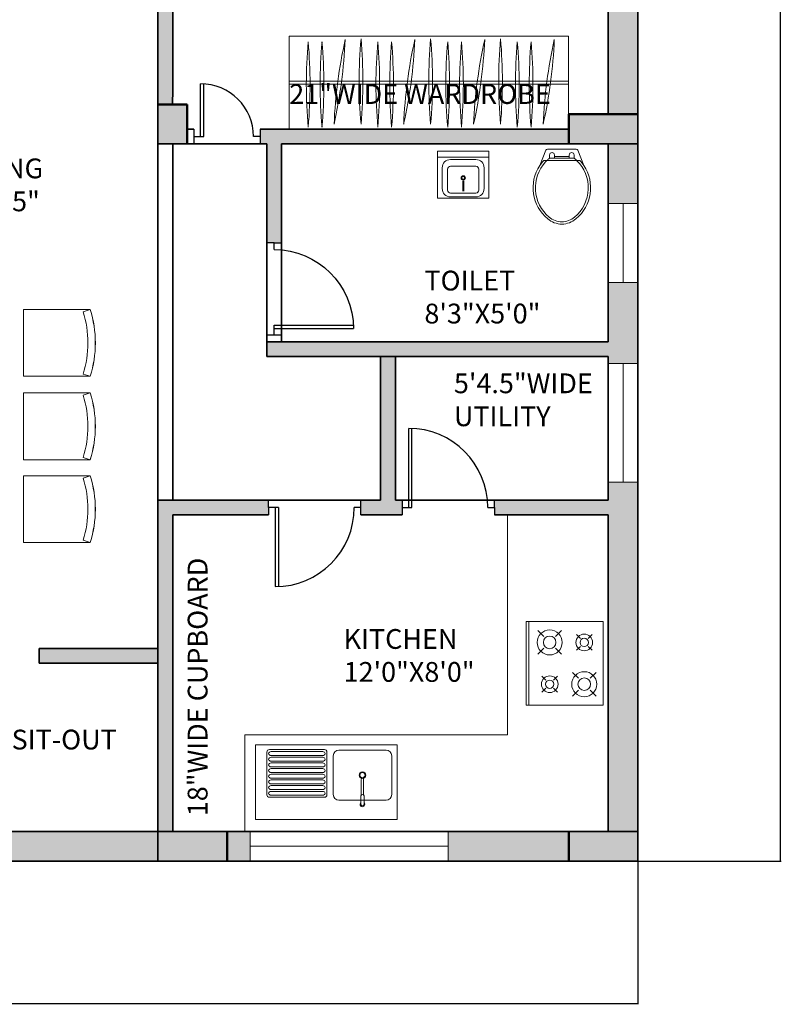
# Model space of a CAD drawing. Units: inches. Extents: x -28 to 485, y -861 to 54.
# Tile 4 of 14: x 254 to 485, y -861 to -563. Entities that reach past the tile are written whole.
import ezdxf

# ---------------------------------------------------------------- set-up
doc = ezdxf.new("R2010")
doc.units = ezdxf.units.IN
doc.header["$MEASUREMENT"] = 0
for name, color, linetype, lineweight in [('A-ANNO-DIMS', 2, 'Continuous', 18), ('A-ANNO-TEXT', 7, 'Continuous', 18), ('A-AREA-IDEN', 7, 'Continuous', 18), ('A-COLS', 7, 'Continuous', 50), ('A-COLS-PATT', 8, 'Continuous', 13), ('A-DOOR', 3, 'Continuous', 25), ('A-EQPM', 9, 'Continuous', 18), ('A-FLOR-CASE', 8, 'Continuous', 18), ('A-FLOR-FIXT', 9, 'Continuous', 18), ('A-FURN', 8, 'Continuous', 13), ('A-GLAZ', 4, 'Continuous', 18), ('A-WALL', 7, 'Continuous', 35), ('A-WALL-PATT', 34, 'Continuous', 13)]:
    doc.layers.add(name, color=color, linetype=linetype, lineweight=lineweight)
doc.styles.get("Standard").update_dxf_attribs({"font": 'arial.ttf'})
doc.dimstyles.get("Standard").update_dxf_attribs({"dimtxt": 0.18, "dimasz": 0.18, "dimexe": 0.18, "dimexo": 0.0625, "dimgap": 0.09, "dimtad": 0, "dimtih": 1, "dimtoh": 1, "dimdec": 0, "dimzin": 0, "dimdsep": 46, "dimlunit": 3, "dimtxsty": 'Standard', "dimcen": 0.09, "dimadec": 0, "dimazin": 0, "dimtfac": 1, "dimtdec": 0, "dimtofl": 0, "dimtmove": 0, "dimatfit": 3, "dimfxl": 1, "dimtolj": 1, "dimtzin": 0, "dimarcsym": 0})

# ---------------------------------------------------------------- blocks, each defined once
blk = doc.blocks.new('М14 600х655')
for p, q in [((-655, 600), (-655, 0)), ((-655, 600), (-655, 0)), ((-655, 0), (-655, 600)), ((0, 600), (-655, 600)), ((0, 525), (-655, 525)), ((0, 0), (0, 600)), ((-596, 388), (-596, 121)), ((-165, 494), (-490, 494)), ((-165, 408), (-490, 408)), ((-59, 121), (-59, 388)), ((-528, 370), (-528, 103)), ((-127, 103), (-127, 370)), ((-334, 87), (-334, 220)), ((-321, 87), (-321, 220)), ((-655, 0), (-655, 0)), ((-655, 0), (-655, 0)), ((-655, 0), (0, 0)), ((-655, 0), (0, 0)), ((-490, 65), (-165, 65)), ((-490, 15), (-165, 15))]:
    blk.add_line(p, q)
for radius in [27.6, 19.3]:
    blk.add_circle((-327, 259), radius)
for centre, radius, start, end in [((-490, 388), 106, 90, 180), ((-490, 370), 38.2, 90, 180), ((-165, 388), 106, 0, 90), ((-165, 370), 38.2, 0, 90), ((-490, 121), 106, 180, 270), ((-490, 103), 38.2, 180, 270), ((-165, 121), 106, 270, 0), ((-165, 103), 38.2, 270, 0)]:
    blk.add_arc(centre, radius, start, end)
blk = doc.blocks.new('WARDROBE-HANGING')
for p, q in [((84.7, 28.23), (0, 28.23)), ((0, 28.23), (0, 0)), ((84.7, 28.23), (84.7, 0)), ((84.7, 14.59), (0, 14.59)), ((84.7, 13.65), (0, 13.65)), ((84.7, 0), (0, 0))]:
    blk.add_line(p, q)
for centre, start, end in [((-131.46, 33.65), 347.508, 357.5023), ((162.01, -4.96), 167.508, 177.5023), ((169.76, 14.46), 175.0028, 184.9972), ((-126.23, 14.46), 355.0028, 4.9972), ((-110.36, 33.65), 347.508, 357.5023), ((183.11, -4.96), 167.508, 177.5023), ((190.86, 14.46), 175.0028, 184.9972), ((-105.13, 14.46), 355.0028, 4.9972), ((204.29, -4.96), 167.508, 177.5023), ((-89.17, 33.65), 347.508, 357.5023), ((212.05, 14.46), 175.0028, 184.9972), ((-83.95, 14.46), 355.0028, 4.9972), ((225.4, -4.96), 167.508, 177.5023), ((-68.07, 33.65), 347.508, 357.5023), ((153.74, 13.55), 175.0028, 184.9972), ((-142.25, 13.55), 355.0028, 4.9972), ((157.93, 13.55), 175.0028, 184.9972), ((-138.07, 13.55), 355.0028, 4.9972), ((174.85, 13.55), 175.0028, 184.9972), ((-121.15, 13.55), 355.0028, 4.9972), ((179.03, 13.55), 175.0028, 184.9972), ((-116.97, 13.55), 355.0028, 4.9972), ((196.03, 13.55), 175.0028, 184.9972), ((-99.97, 13.55), 355.0028, 4.9972), ((200.21, 13.55), 175.0028, 184.9972), ((-95.78, 13.55), 355.0028, 4.9972), ((217.13, 13.55), 175.0028, 184.9972), ((-78.86, 13.55), 355.0028, 4.9972), ((221.31, 13.55), 175.0028, 184.9972), ((-74.68, 13.55), 355.0028, 4.9972)]:
    blk.add_arc(centre, 148.56, start, end)
blk = doc.blocks.new('WC-FLOOR-MOUNTED')
for p, q in [((3.27, 19.35), (4.23, 19.35)), ((4.23, 19.35), (8.71, 19.35)), ((13.2, 19.35), (8.71, 19.35)), ((13.2, 19.35), (14.16, 19.35))]:
    blk.add_line(p, q)
for points in [[(8.71, 22.81), (4.36, 22.81, 0.31031), (3.82, 22.44), (2.03, 17.79, 0.209071)], [(5.01, 20.04), (5.01, 21, -1), (6.47, 21), (6.47, 20.5)], [(8.71, 22.81), (13.07, 22.81, -0.31031), (13.6, 22.44), (15.39, 17.79, -0.209071)], [(12.41, 20.04), (12.41, 21, 1), (10.96, 21), (10.96, 20.5)], [(3.77, 18.89, 0.431639), (4.86, 2.17, 0.162618), (8.71, 0.68, 0.470877)], [(3.27, 19.35, 0.040937), (2.03, 17.79, 0.163732)], [(4.23, 19.35, 0.014165), (3.77, 18.89, 0.162618)], [(5.01, 20.04, 0.022712), (4.23, 19.35, 0.162618)], [(8.71, 20.04), (5.01, 20.04, 0.022712)], [(8.71, 20.04), (12.41, 20.04, -0.476108)], [(13.2, 19.35, -0.448546), (12.57, 2.17, -0.162618), (8.71, 0.68, -0.470877)], [(12.41, 20.04, -0.022712), (13.2, 19.35, -0.162618)], [(14.16, 19.35, -0.040937), (15.39, 17.79, -0.163732)], [(2.03, 17.79, 0.383919), (4.43, 1.64, 0.163732), (8.71, 0, 0.359733)], [(15.39, 17.79, -0.383919), (13, 1.64, -0.163732), (8.71, 0, -0.359733)]]:
    blk.add_lwpolyline(points, format="xyb")
for points in [[(10.96, 20.5), (6.47, 20.5)], [(6.47, 20.5), (6.47, 20.04)], [(10.96, 20.5), (10.96, 20.04)]]:
    blk.add_lwpolyline(points)
blk = doc.blocks.new('COOKTOP-FOUR-BURNER')
for p, q in [((0, 0), (0, 25.33)), ((0, 25.33), (23.39, 25.33)), ((0.84, 0), (0.84, 25.33)), ((23.39, 0), (23.39, 25.33)), ((5.39, 20.79), (3.59, 22.58)), ((8.97, 20.79), (10.76, 22.58)), ((16.47, 20.19), (15.27, 21.39)), ((18.85, 20.19), (20.05, 21.39)), ((5.39, 17.21), (3.59, 15.42)), ((8.97, 17.21), (10.76, 15.42)), ((16.47, 17.8), (15.27, 16.61)), ((18.85, 17.8), (20.05, 16.61)), ((15.87, 8.12), (14.08, 9.91)), ((19.45, 8.12), (21.24, 9.91)), ((5.98, 7.53), (4.79, 8.72)), ((8.37, 7.53), (9.57, 8.72)), ((5.98, 5.14), (4.79, 3.94)), ((8.37, 5.14), (9.57, 3.94)), ((15.87, 4.54), (14.08, 2.75)), ((19.45, 4.54), (21.24, 2.75)), ((0, 0), (23.39, 0))]:
    blk.add_line(p, q)
for centre, radius in [((7.18, 19), 3.8), ((17.66, 19), 2.53), ((17.66, 6.33), 3.8), ((7.18, 6.33), 2.53)]:
    blk.add_circle(centre, radius)
for centre, radius, start, end in [((7.18, 19), 1.9, 90, 270), ((7.18, 19), 1.9, 270, 90), ((17.66, 19), 1.27, 90, 270), ((17.66, 19), 1.27, 270, 90), ((7.18, 6.33), 1.27, 90, 270), ((7.18, 6.33), 1.27, 270, 90), ((17.66, 6.33), 1.9, 90, 270), ((17.66, 6.33), 1.9, 270, 90)]:
    blk.add_arc(centre, radius, start, end)
blk = doc.blocks.new('CHAIR-DINING')
for p, q in [((20.22, 20.23), (18.08, 19.55)), ((20.22, 0), (18.08, 0.68))]:
    blk.add_line(p, q)
blk.add_lwpolyline([(20.23, 0), (0, 0), (0, 20.23), (20.23, 20.23, -0.153703), (20.23, 0)], format="xyb")
for radius in [31.13, 33.37]:
    blk.add_arc((-11.59, 10.12), radius, 342.3544, 17.6456)
blk = doc.blocks.new('DOOR-SWING-24')
for p, q in [((2, 2.25), (2, 26.25)), ((3, 2.25), (3, 26.25)), ((0, 4.5), (0, 0)), ((28, 2.25), (28, 4.5)), ((0, 2.25), (2, 2.25)), ((2, 2.25), (3, 2.25)), ((26, 2.25), (28, 2.25)), ((28, 2.25), (28, 0))]:
    blk.add_line(p, q)
blk.add_arc((2, 2.25), 24, 0, 90)
blk = doc.blocks.new('DOOR-SWING-KITCHEN')
for p, q in [((0, 24), (0, 26.25)), ((2, 24), (0, 24)), ((0, 24), (0, 21.75)), ((2, 24), (2, 0)), ((3, 24), (2, 24)), ((3, 24), (3, 0)), ((28, 24), (26, 24)), ((28, 21.75), (28, 26.25))]:
    blk.add_line(p, q)
blk.add_arc((2, 24), 24, 270, 0)
blk = doc.blocks.new('WINDOW-60IN')
for p, q in [((0, 60), (0, 0)), ((9, 60), (0, 60)), ((4.5, 60), (4.5, 0)), ((9, 0), (9, 60)), ((0, 0), (9, 0))]:
    blk.add_line(p, q)
blk = doc.blocks.new('WINDOW-36IN')
for p, q in [((0, 36), (0, 0)), ((9, 36), (0, 36)), ((4.5, 36), (4.5, 0)), ((9, 0), (9, 36)), ((0, 0), (9, 0))]:
    blk.add_line(p, q)
blk = doc.blocks.new('WINDOW-24IN')
for p, q in [((0, 24), (0, 0)), ((9, 24), (0, 24)), ((4.5, 24), (4.5, 0)), ((9, 0), (9, 24)), ((9, 0), (0, 0))]:
    blk.add_line(p, q)
blk = doc.blocks.new('*D52')
at = {"layer": 'A-ANNO-DIMS', "color": 0, "lineweight": -2, "transparency": 16777216}
for p, q in [((15.28, -817.93), (15.28, -861.3)), ((441.28, -817.93), (441.28, -861.3)), ((15.46, -861.12), (227.99, -861.12)), ((441.1, -861.12), (228.58, -861.12))]:
    blk.add_line(p, q, dxfattribs=at)
at = {"layer": 'A-ANNO-DIMS', "color": 0, "transparency": 16777216}
for points in [[(15.46, -861.09), (15.46, -861.15), (15.28, -861.12)], [(441.1, -861.09), (441.1, -861.15), (441.28, -861.12)]]:
    blk.add_solid(points, dxfattribs=at)
at = {"layer": 'Defpoints', "color": 0, "transparency": 16777216}
for p in [(15.28, -817.87), (441.28, -817.87), (441.28, -861.12)]:
    blk.add_point(p, dxfattribs=at)
at = {"layer": 'A-ANNO-DIMS', "color": 0, "transparency": 16777216, "insert": (228.28, -861.12), "char_height": 0.18, "attachment_point": 5}
blk.add_mtext('\\A1;426', dxfattribs=at)
blk = doc.blocks.new('*D53')
at = {"layer": 'A-ANNO-DIMS', "color": 0, "lineweight": -2, "transparency": 16777216}
for p, q in [((441.35, 10.13), (484.71, 10.13)), ((484.53, 9.95), (484.53, -403.68)), ((484.53, -817.69), (484.53, -404.05)), ((441.35, -817.87), (484.71, -817.87))]:
    blk.add_line(p, q, dxfattribs=at)
at = {"layer": 'A-ANNO-DIMS', "color": 0, "transparency": 16777216}
for points in [[(484.5, 9.95), (484.56, 9.95), (484.53, 10.13)], [(484.5, -817.69), (484.56, -817.69), (484.53, -817.87)]]:
    blk.add_solid(points, dxfattribs=at)
at = {"layer": 'Defpoints', "color": 0, "transparency": 16777216}
for p in [(441.28, 10.13), (441.28, -817.87), (484.53, -817.87)]:
    blk.add_point(p, dxfattribs=at)
at = {"layer": 'A-ANNO-DIMS', "color": 0, "transparency": 16777216, "insert": (484.53, -403.87), "char_height": 0.18, "attachment_point": 5}
blk.add_mtext('\\A1;828', dxfattribs=at)

msp = doc.modelspace()

# ---------------------------------------------------------------- hatches: boundary and pattern name
at = {"layer": 'A-COLS-PATT'}
h = msp.add_hatch(color=256, dxfattribs=at)
h.dxf.hatch_style = 1
h.paths.add_polyline_path([(441.285, -591.367), (420.285, -591.367), (420.285, -595.867), (420.285, -600.367), (441.285, -600.367)])
h.paths.add_polyline_path([(304.691, -588.367), (295.785, -588.367), (295.785, -600.367), (304.691, -600.367)])
h.paths.add_polyline_path([(160.785, -588.367), (151.785, -588.367), (151.785, -600.367), (160.785, -600.367)])
h.paths.add_polyline_path([(36.285, -591.367), (24.285, -591.367), (15.285, -591.367), (15.285, -600.367), (36.285, -600.367)])
h.paths.add_polyline_path([(36.285, -808.867), (15.285, -808.867), (15.285, -817.867), (36.285, -817.867)])
h.paths.add_polyline_path([(160.785, -808.867), (139.785, -808.867), (139.785, -817.867), (160.785, -817.867)])
h.paths.add_polyline_path([(316.785, -808.867), (295.785, -808.867), (295.785, -817.867), (316.785, -817.867)])
h.paths.add_polyline_path([(441.285, -808.867), (420.285, -808.867), (420.285, -817.867), (441.285, -817.867)])
h.paths.add_polyline_path([(36.285, -442.867), (15.285, -442.867), (15.285, -451.867), (36.285, -451.867)])
h.paths.add_polyline_path([(160.785, -442.867), (139.785, -442.867), (139.785, -451.867), (160.785, -451.867)])
h.paths.add_polyline_path([(316.785, -442.867), (295.785, -442.867), (295.785, -451.867), (316.785, -451.867)])
h.paths.add_polyline_path([(441.285, -442.867), (420.285, -442.867), (420.285, -451.867), (441.285, -451.867)])
at = {"layer": 'A-WALL-PATT'}
h = msp.add_hatch(color=256, dxfattribs=at)
h.dxf.hatch_style = 1
h.paths.add_polyline_path([(160.785, -808.867), (160.785, -817.867), (295.785, -817.867), (295.785, -808.867)])
h.paths.add_polyline_path([(316.785, -817.867), (323.776, -817.867), (323.776, -808.867), (316.785, -808.867)])
h.paths.add_polyline_path([(420.285, -817.867), (420.285, -808.867), (383.776, -808.867), (383.776, -817.867)])
h.paths.add_polyline_path([(432.285, -808.867), (441.285, -808.867), (441.285, -702.966), (432.285, -702.966), (432.285, -708.367), (397.785, -708.367), (397.785, -710.617), (397.785, -712.867), (432.285, -712.867)])
h.paths.add_polyline_path([(300.285, -712.867), (329.285, -712.867), (329.285, -710.617), (329.285, -708.367), (295.785, -708.367), (295.785, -808.867), (300.285, -808.867)])
h.paths.add_polyline_path([(160.785, -698.867), (158.535, -698.867), (156.285, -698.867), (156.285, -808.867), (160.785, -808.867)])
h.paths.add_polyline_path([(36.285, -808.867), (36.285, -817.867), (79.721, -817.867), (79.721, -808.867)])
h.paths.add_polyline_path([(15.285, -808.867), (24.285, -808.867), (24.285, -739.09), (15.285, -739.09)])
h.paths.add_polyline_path([(24.285, -640.781), (15.285, -640.781), (15.285, -679.09), (24.285, -679.09), (24.285, -664.867), (89.285, -664.867), (89.285, -662.617), (89.285, -660.367), (24.285, -660.367)])
h.paths.add_polyline_path([(15.285, -616.781), (24.285, -616.781), (24.285, -600.367), (15.285, -600.367)])
h.paths.add_polyline_path([(36.285, -595.867), (36.285, -600.367), (123.285, -600.367), (123.285, -660.367), (117.285, -660.367), (117.285, -664.867), (156.285, -664.867), (156.285, -670.867), (160.785, -670.867), (160.785, -660.367), (127.785, -660.367), (127.785, -600.367), (129.785, -600.367), (129.785, -598.117), (129.785, -595.867)])
h.paths.add_polyline_path([(367.785, -664.867), (363.285, -664.867), (363.285, -708.367), (357.285, -708.367), (357.285, -712.867), (369.785, -712.867), (369.785, -708.367), (367.785, -708.367)])
h.paths.add_polyline_path([(432.285, -664.867), (432.285, -666.966), (441.285, -666.966), (441.285, -642.367), (432.285, -642.367), (432.285, -660.367), (328.785, -660.367), (328.785, -664.867), (363.285, -664.867)])
h.paths.add_polyline_path([(333.285, -600.367), (420.285, -600.367), (420.285, -595.867), (326.785, -595.867), (326.785, -600.367), (328.785, -600.367), (328.785, -630.367), (331.035, -630.367), (333.285, -630.367)])
h.paths.add_polyline_path([(441.285, -600.367), (432.285, -600.367), (432.285, -618.367), (441.285, -618.367)])
h.paths.add_polyline_path([(432.285, -591.367), (441.285, -591.367), (441.285, -547.793), (432.285, -547.793)])
h.paths.add_polyline_path([(295.785, -588.367), (300.238, -588.367), (300.285, -583.867), (300.285, -451.867), (295.785, -451.867)])
h.paths.add_polyline_path([(420.285, -451.867), (420.285, -442.867), (316.785, -442.867), (316.785, -451.867)])
h.paths.add_polyline_path([(432.285, -487.793), (441.285, -487.793), (441.285, -451.867), (432.285, -451.867)])
h.paths.add_polyline_path([(432.285, -442.867), (441.285, -442.867), (441.285, -364.867), (432.285, -364.867)])
h.paths.add_polyline_path([(261.785, -451.867), (261.785, -447.367), (261.785, -444.758), (261.785, -442.867), (160.785, -442.867), (160.785, -451.867)])
h.paths.add_polyline_path([(139.785, -451.867), (139.785, -442.867), (36.285, -442.867), (36.285, -451.867)])
h.paths.add_polyline_path([(15.285, -491.617), (24.285, -491.617), (24.285, -451.867), (15.285, -451.867)])
h.paths.add_polyline_path([(24.285, -551.617), (15.285, -551.617), (15.285, -591.367), (24.285, -591.367)])
h.paths.add_polyline_path([(160.785, -451.867), (156.285, -451.867), (156.285, -588.367), (160.785, -588.367)])
h.paths.add_polyline_path([(139.785, -364.867), (139.785, -355.867), (36.285, -355.867), (36.285, -364.867)])
h.paths.add_polyline_path([(24.285, -364.867), (15.285, -364.867), (15.285, -373.867), (24.285, -373.867)])
h.paths.add_polyline_path([(15.285, -433.867), (15.285, -442.867), (24.285, -442.867), (24.285, -433.867)])
h.paths.add_polyline_path([(261.785, -364.867), (261.785, -360.367), (261.785, -355.867), (160.785, -355.867), (160.785, -364.867)])
h.paths.add_polyline_path([(295.785, -355.867), (289.785, -355.867), (289.785, -364.867), (295.785, -364.867)])
h.paths.add_polyline_path([(295.785, -355.867), (300.285, -355.867), (300.285, -259.867), (333.285, -259.867), (333.285, -257.617), (333.285, -255.367), (300.285, -255.367), (300.285, -207.367), (295.785, -207.367)])
h.paths.add_polyline_path([(420.285, -364.867), (420.285, -355.867), (316.785, -355.867), (316.785, -364.867)])
h.paths.add_polyline_path([(24.285, -311.192), (15.285, -311.192), (15.285, -355.867), (24.285, -355.867)])
h.paths.add_polyline_path([(24.285, -211.867), (54.144, -211.867), (54.144, -207.367), (24.285, -207.367), (24.285, -187.772), (15.285, -187.772), (15.285, -251.192), (24.285, -251.192)])
h.paths.add_polyline_path([(82.144, -207.367), (82.144, -209.617), (82.144, -211.867), (127.785, -211.867), (127.785, -147.367), (129.785, -147.367), (129.785, -145.117), (129.785, -142.867), (36.285, -142.867), (36.285, -147.367), (123.285, -147.367), (123.285, -207.367)])
h.paths.add_polyline_path([(160.785, -207.367), (156.285, -207.367), (156.285, -355.867), (160.785, -355.867)])
h.paths.add_polyline_path([(24.285, 1.133), (15.285, 1.133), (15.285, -54.408), (24.285, -54.408)])
h.paths.add_polyline_path([(36.285, 10.133), (36.285, 1.133), (70.235, 1.133), (70.235, 10.133)])
h.paths.add_polyline_path([(15.285, -138.367), (24.285, -138.367), (24.285, -114.408), (15.285, -114.408)])
h.paths.add_polyline_path([(24.285, -147.367), (15.285, -147.367), (15.285, -163.772), (24.285, -163.772)])
h.paths.add_polyline_path([(156.285, -130.867), (160.785, -130.867), (160.785, 1.133), (156.285, 1.133)])
h.paths.add_polyline_path([(130.235, 1.133), (139.785, 1.133), (139.785, 10.133), (130.235, 10.133)])
h.paths.add_polyline_path([(316.785, 10.133), (316.785, 1.133), (328.097, 1.133), (328.097, 10.133)])
h.paths.add_polyline_path([(300.285, 1.133), (295.785, 1.133), (295.785, -130.867), (300.285, -130.867)])
h.paths.add_polyline_path([(420.285, -147.367), (420.285, -142.867), (326.785, -142.867), (326.785, -145.117), (326.785, -147.367), (328.785, -147.367), (328.785, -177.367), (331.035, -177.367), (333.285, -177.367), (333.285, -147.367)])
h.paths.add_polyline_path([(333.285, -207.367), (333.285, -205.367), (328.785, -205.367), (328.785, -211.867), (363.285, -211.867), (363.285, -255.367), (361.285, -255.367), (361.285, -259.867), (369.785, -259.867), (369.785, -255.367), (367.785, -255.367), (367.785, -211.867), (432.285, -211.867), (432.285, -214.893), (441.285, -214.893), (441.285, -188.008), (432.285, -188.008), (432.285, -207.367)])
h.paths.add_polyline_path([(441.285, -250.893), (432.285, -250.893), (432.285, -255.367), (397.785, -255.367), (397.785, -257.617), (397.785, -259.867), (432.285, -259.867), (432.285, -355.867), (441.285, -355.867)])
h.paths.add_polyline_path([(432.285, -138.367), (441.285, -138.367), (441.285, -115.099), (432.285, -115.099)])
h.paths.add_polyline_path([(441.285, -147.367), (432.285, -147.367), (432.285, -164.008), (441.285, -164.008)])
h.paths.add_polyline_path([(420.285, 1.133), (420.285, 10.133), (388.097, 10.133), (388.097, 1.133)])
h.paths.add_polyline_path([(432.285, -55.099), (441.285, -55.099), (441.285, 1.133), (432.285, 1.133)])
h = msp.add_hatch(color=256, dxfattribs=at)
h.dxf.hatch_style = 1
h.paths.add_polyline_path([(196.785, -58.867), (160.785, -58.867), (160.785, -63.367), (196.785, -63.367)])
h.paths.add_polyline_path([(295.785, -58.867), (259.785, -58.867), (259.785, -63.367), (295.785, -63.367)])
h.paths.add_polyline_path([(196.785, -753.367), (160.785, -753.367), (160.785, -757.867), (196.785, -757.867)])
h.paths.add_polyline_path([(295.785, -753.367), (259.785, -753.367), (259.785, -757.867), (295.785, -757.867)])

# ---------------------------------------------------------------- linework, layer by layer
at = {"layer": 'A-COLS'}
for p, q in [((304.691, -588.367), (295.785, -588.367)), ((304.691, -600.367), (304.691, -588.367)), ((420.285, -595.867), (420.285, -591.367)), ((420.285, -591.367), (441.285, -591.367)), ((420.285, -600.367), (420.285, -595.867)), ((316.785, -808.867), (316.785, -817.867)), ((420.285, -808.867), (420.285, -817.867))]:
    msp.add_line(p, q, dxfattribs=at)
at = {"layer": 'A-DOOR'}
for p, q in [((308.691, -598.117), (308.691, -582.117)), ((309.691, -598.117), (309.691, -582.117)), ((306.691, -595.867), (306.691, -600.367)), ((326.785, -595.867), (326.785, -600.367)), ((306.691, -598.117), (308.691, -598.117)), ((308.691, -598.117), (309.691, -598.117)), ((326.785, -598.117), (324.785, -598.117))]:
    msp.add_line(p, q, dxfattribs=at)
msp.add_arc((308.691, -598.211), 16.094, 0.33541, 90, dxfattribs=at)
at = {"layer": 'A-FLOR-CASE'}
for p, q in [((401.695, -712.867), (401.695, -779.545)), ((401.695, -779.545), (322.083, -779.545)), ((322.083, -779.545), (322.083, -808.867))]:
    msp.add_line(p, q, dxfattribs=at)
at = {"layer": 'A-FLOR-FIXT'}
for p, q in [((368.283, -782.631), (325.404, -782.631)), ((325.404, -782.631), (325.404, -805.296)), ((328.806, -797.721), (328.806, -784.819)), ((346.232, -784.037), (329.587, -784.037)), ((337.91, -784.659), (330.057, -784.659)), ((337.91, -784.659), (345.762, -784.659)), ((347.014, -797.721), (347.014, -784.819)), ((364.954, -784.208), (350.618, -784.208)), ((368.283, -782.631), (368.283, -805.296)), ((337.91, -785.831), (330.057, -785.831)), ((337.91, -786.38), (330.057, -786.38)), ((337.91, -787.552), (330.057, -787.552)), ((337.91, -788.101), (330.057, -788.101)), ((337.91, -785.831), (345.762, -785.831)), ((337.91, -786.38), (345.762, -786.38)), ((337.91, -787.552), (345.762, -787.552)), ((337.91, -788.101), (345.762, -788.101)), ((348.93, -785.896), (348.93, -797.675)), ((366.642, -797.675), (366.642, -785.896)), ((337.91, -789.273), (330.057, -789.273)), ((337.91, -789.821), (330.057, -789.821)), ((337.91, -790.993), (330.057, -790.993)), ((337.91, -789.273), (345.762, -789.273)), ((337.91, -789.821), (345.762, -789.821)), ((337.91, -790.993), (345.762, -790.993)), ((337.91, -791.542), (330.057, -791.542)), ((337.91, -792.714), (330.057, -792.714)), ((337.91, -793.263), (330.057, -793.263)), ((337.91, -791.542), (345.762, -791.542)), ((337.91, -792.714), (345.762, -792.714)), ((337.91, -793.263), (345.762, -793.263)), ((337.91, -794.435), (330.057, -794.435)), ((337.91, -794.984), (330.057, -794.984)), ((337.91, -796.156), (330.057, -796.156)), ((337.91, -796.705), (330.057, -796.705)), ((337.91, -794.435), (345.762, -794.435)), ((337.91, -794.984), (345.762, -794.984)), ((337.91, -796.156), (345.762, -796.156)), ((337.91, -796.705), (345.762, -796.705)), ((329.587, -798.503), (346.232, -798.503)), ((337.91, -797.877), (330.057, -797.877)), ((337.91, -797.877), (345.762, -797.877)), ((350.618, -799.363), (357.317, -799.363)), ((357.525, -799.363), (364.954, -799.363)), ((368.283, -805.296), (325.404, -805.296))]:
    msp.add_line(p, q, dxfattribs=at)
for points in [[(357.434, -797.812), (357.434, -793.067)], [(358.138, -797.812), (358.138, -793.067)], [(357.317, -800.68), (357.317, -798.104)], [(358.255, -800.68), (358.255, -798.104)]]:
    msp.add_lwpolyline(points, dxfattribs=at)
for radius in [0.977, 0.782]:
    msp.add_circle((357.786, -791.786), radius, dxfattribs=at)
for centre, radius, start, end in [((329.587, -784.819), 0.782, 90, 180), ((330.057, -785.44), 0.782, 90, 165.50967), ((330.057, -785.049), 0.782, 194.49033, 270), ((345.762, -785.44), 0.782, 14.49033, 90), ((345.762, -785.049), 0.782, 270, 345.50967), ((346.232, -784.819), 0.782, 0, 90), ((350.618, -785.896), 1.688, 90, 180), ((364.954, -785.896), 1.688, 0, 90), ((330.057, -787.161), 0.782, 90, 165.50967), ((330.057, -786.77), 0.782, 194.49033, 270), ((330.057, -788.882), 0.782, 90, 165.50967), ((345.762, -787.161), 0.782, 14.49033, 90), ((345.762, -786.77), 0.782, 270, 345.50967), ((345.762, -788.882), 0.782, 14.49033, 90), ((330.057, -788.491), 0.782, 194.49033, 270), ((330.057, -790.603), 0.782, 90, 165.50967), ((330.057, -790.212), 0.782, 194.49033, 270), ((345.762, -788.491), 0.782, 270, 345.50967), ((345.762, -790.603), 0.782, 14.49033, 90), ((345.762, -790.212), 0.782, 270, 345.50967), ((330.057, -792.324), 0.782, 90, 165.50967), ((330.057, -791.933), 0.782, 194.49033, 270), ((330.057, -794.045), 0.782, 90, 165.50967), ((330.057, -793.654), 0.782, 194.49033, 270), ((345.762, -792.324), 0.782, 14.49033, 90), ((345.762, -791.933), 0.782, 270, 345.50967), ((345.762, -794.045), 0.782, 14.49033, 90), ((345.762, -793.654), 0.782, 270, 345.50967), ((357.786, -793.036), 0.353, 354.94633, 185.05367), ((330.057, -795.766), 0.782, 90, 165.50967), ((330.057, -795.374), 0.782, 194.49033, 270), ((330.057, -797.486), 0.782, 90, 165.50967), ((330.057, -797.095), 0.782, 194.49033, 270), ((345.762, -795.766), 0.782, 14.49033, 90), ((345.762, -795.374), 0.782, 270, 345.50967), ((345.762, -797.486), 0.782, 14.49033, 90), ((345.762, -797.095), 0.782, 270, 345.50967), ((329.587, -797.721), 0.782, 180, 270), ((346.232, -797.721), 0.782, 270, 0), ((350.618, -797.675), 1.688, 180, 270), ((357.786, -800.68), 0.702, 131.90178, 48.09822), ((357.786, -798.123), 0.469, 2.21976, 177.78024), ((364.954, -797.675), 1.688, 270, 0), ((357.786, -800.68), 0.469, 180, 0)]:
    msp.add_arc(centre, radius, start, end, dxfattribs=at)
at = {"layer": 'A-WALL'}
for p, q in [((441.285, 10.133), (441.285, -817.867)), ((295.785, -442.867), (295.785, -817.867)), ((300.285, -451.867), (300.285, -583.867)), ((432.285, -451.867), (432.285, -591.367)), ((300.285, -583.867), (300.238, -588.367)), ((304.785, -595.867), (304.691, -595.867)), ((304.785, -595.867), (306.691, -595.867)), ((326.785, -595.867), (420.285, -595.867)), ((295.785, -600.367), (328.785, -600.367)), ((300.285, -600.367), (300.285, -660.367)), ((328.785, -600.367), (328.785, -660.367)), ((333.285, -600.367), (333.285, -660.367)), ((333.285, -600.367), (441.285, -600.367)), ((432.285, -600.367), (432.285, -660.367)), ((328.785, -664.867), (328.785, -658.367)), ((300.285, -660.367), (300.285, -664.867)), ((328.785, -660.367), (432.285, -660.367)), ((300.285, -664.867), (300.285, -708.367)), ((363.285, -664.867), (328.785, -664.867)), ((363.285, -664.867), (432.285, -664.867)), ((363.285, -664.867), (363.285, -708.367)), ((367.785, -664.867), (367.785, -708.367)), ((432.285, -664.867), (432.285, -708.367)), ((295.785, -708.367), (363.285, -708.367)), ((367.785, -708.367), (432.285, -708.367)), ((300.285, -712.867), (329.285, -712.867)), ((300.285, -712.867), (300.285, -808.867)), ((357.285, -712.867), (369.785, -712.867)), ((397.785, -712.867), (432.285, -712.867)), ((432.285, -712.867), (432.285, -808.867)), ((259.785, -753.367), (259.785, -757.867)), ((259.785, -753.367), (295.785, -753.367)), ((259.785, -757.867), (295.785, -757.867)), ((15.285, -808.867), (441.285, -808.867)), ((15.285, -817.867), (441.285, -817.867))]:
    msp.add_line(p, q, dxfattribs=at)

# ---------------------------------------------------------------- block references
at = {"layer": 'A-DOOR', "extrusion": (0, 0, -1), "zscale": -1, "rotation": 90}
msp.add_blockref('DOOR-SWING-24', (-328.785, -658.367), dxfattribs=at)
at = {"layer": 'A-DOOR'}
for name, p in [('DOOR-SWING-24', (369.785, -712.867)), ('DOOR-SWING-KITCHEN', (329.285, -734.617))]:
    msp.add_blockref(name, p, dxfattribs=at)
at = {"layer": 'A-EQPM'}
msp.add_blockref('COOKTOP-FOUR-BURNER', (407.353, -770.539), dxfattribs=at)
at = {"layer": 'A-FLOR-CASE'}
msp.add_blockref('WARDROBE-HANGING', (335.582, -595.867), dxfattribs=at)
at = {"layer": 'A-FLOR-FIXT', "xscale": 0.0236562783211592, "yscale": 0.0236562783211592, "zscale": 0.0236562783211592}
msp.add_blockref('М14 600х655', (396.058, -616.771), dxfattribs=at)
at = {"layer": 'A-FLOR-FIXT'}
msp.add_blockref('WC-FLOOR-MOUNTED', (409.503, -624.705), dxfattribs=at)
at = {"layer": 'A-FURN'}
for p in [(255.021, -670.816), (255.021, -696.113), (255.021, -721.245)]:
    msp.add_blockref('CHAIR-DINING', p, dxfattribs=at)
at = {"layer": 'A-GLAZ'}
for name, p in [('WINDOW-24IN', (432.285, -642.367)), ('WINDOW-36IN', (432.285, -702.966))]:
    msp.add_blockref(name, p, dxfattribs=at)
at = {"layer": 'A-GLAZ', "rotation": 90}
msp.add_blockref('WINDOW-60IN', (383.775, -817.867), dxfattribs=at)

# ---------------------------------------------------------------- texts
at = {"layer": 'A-ANNO-TEXT', "insert": (335.581, -582.22), "char_height": 6, "attachment_point": 1}
msp.add_mtext('21"WIDE WARDROBE', dxfattribs=at)
at = {"layer": 'A-ANNO-TEXT', "insert": (304.809, -804.245), "char_height": 6, "attachment_point": 1, "rotation": 90}
msp.add_mtext('18"WIDE CUPBOARD', dxfattribs=at)
at = {"layer": 'A-AREA-IDEN', "char_height": 6, "attachment_point": 1}
for s, insert in [('LIVING/DINING\\P11\'3"X25\'10.5"', (204.363, -604.771)), ('TOILET\\P8\'3"X5\'0"', (376.557, -638.798)), ('5\'4.5"WIDE\\PUTILITY', (385.499, -669.955)), ('KITCHEN\\P12\'0"X8\'0"', (352.061, -747.489)), ('5\'0" WIDE SIT-OUT', (212.472, -778.001))]:
    msp.add_mtext(s, dxfattribs=dict(at, insert=insert))

# ---------------------------------------------------------------- dimensions: what is measured, and where the dimension line sits
at = {"layer": 'A-ANNO-DIMS'}
dim = msp.add_linear_dim(base=(484.535, -817.867), p1=(441.285, 10.133), p2=(441.285, -817.867), angle=90, dimstyle='Standard', override={"dimdec": 0, "dimlfac": 1, "dimrnd": 0, "dimzin": 0, "dimdsep": 46, "dimlunit": 2}, dxfattribs=at)
dim.commit()
dim.dimension.update_dxf_attribs({"geometry": '*D53', "text_midpoint": (484.535, -403.867)})
dim = msp.add_linear_dim(base=(441.285, -861.117), p1=(15.285, -817.867), p2=(441.285, -817.867), dimstyle='Standard', override={"dimdec": 0, "dimlfac": 1, "dimrnd": 0, "dimzin": 0, "dimdsep": 46, "dimlunit": 2}, dxfattribs=at)
dim.commit()
dim.dimension.update_dxf_attribs({"geometry": '*D52', "text_midpoint": (228.285, -861.117)})

doc.saveas('drawing.dxf')
